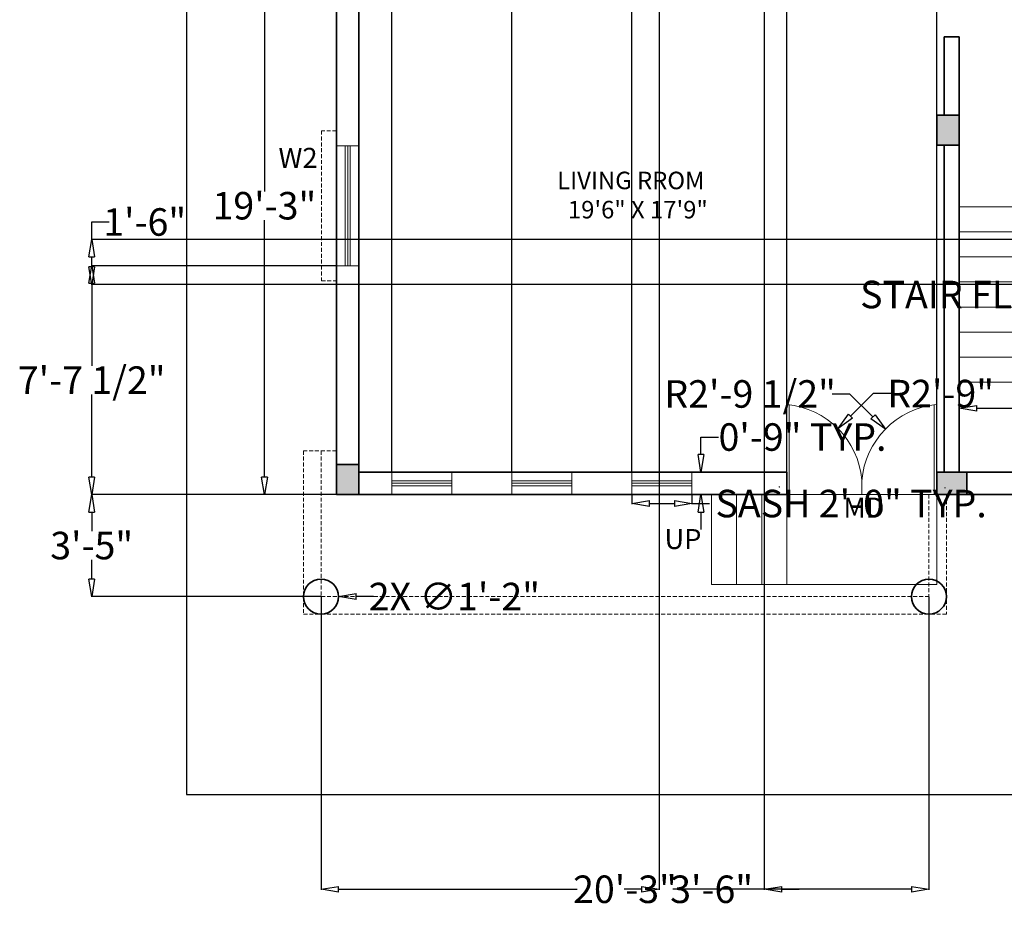
# Model space of a CAD drawing. Units: inches. Extents: x 668 to 1552, y 994 to 1684.
# Tile 1 of 4: x 668 to 1061, y 994 to 1349. Entities that reach past the tile are written whole.
import ezdxf

# ---------------------------------------------------------------- set-up
doc = ezdxf.new("R2010")
doc.units = ezdxf.units.IN
doc.header["$LTSCALE"] = 2.5
doc.header["$MEASUREMENT"] = 0
doc.linetypes.add('HIDDEN', pattern=[0.375, 0.25, -0.125])
for name, color, linetype, lineweight, true_color in [('A-ANNO-DIMS', 175, 'Continuous', 13, 0x4554a5), ('A-ANNO-TEXT', 52, 'Continuous', 18, 0xc8c92d), ('A-DOOR', 152, 'Continuous', 18, 0x2776bb), ('A-FLOR-STRS', 165, 'Continuous', 18, 0x5e67af)]:
    doc.layers.add(name, color=color, linetype=linetype, lineweight=lineweight, true_color=true_color)
for name, color, linetype, lineweight in [('A-AREA-IDEN', 2, 'Continuous', 18), ('A-COLS', 7, 'Continuous', 35), ('A-COLS-PATT', 1, 'Continuous', 13), ('A-GLAZ', 4, 'Continuous', 18), ('A-ROOF-OVHD', 82, 'HIDDEN', 13), ('A-WALL', 7, 'Continuous', 35), ('C-PROP', 1, 'Continuous', 25), ('sajjas', 210, 'HIDDEN', 13)]:
    doc.layers.add(name, color=color, linetype=linetype, lineweight=lineweight)
doc.styles.get("Standard").update_dxf_attribs({"font": 'arial.ttf'})
doc.dimstyles.get("Standard").update_dxf_attribs({"dimtxt": 11, "dimasz": 7, "dimexe": 0.18, "dimexo": 0.0625, "dimgap": 0.09, "dimtad": 0, "dimtih": 1, "dimtoh": 1, "dimdec": 0, "dimzin": 0, "dimdsep": 46, "dimlunit": 3, "dimtxsty": 'Standard', "dimblk": 'CLOSEDBLANK', "dimcen": 0.09, "dimadec": 0, "dimazin": 0, "dimtfac": 1, "dimtdec": 0, "dimtofl": 0, "dimtmove": 0, "dimatfit": 3, "dimldrblk": 'CLOSEDBLANK', "dimfxl": 1, "dimtolj": 1, "dimtzin": 0, "dimarcsym": 0})

# ---------------------------------------------------------------- blocks, each defined once
blk = doc.blocks.new('_ClosedBlank')
at = {"color": 0, "linetype": 'ByBlock', "lineweight": -2}
for p, q in [((-1, 0.167), (0, 0)), ((-1, 0.167), (-1, -0.167)), ((0, 0), (-1, -0.167))]:
    blk.add_line(p, q, dxfattribs=at)
blk = doc.blocks.new('*D5')
at = {"layer": 'A-ANNO-DIMS', "color": 0, "lineweight": -2, "ltscale": 2.5, "transparency": 16777216}
for p, q in [((794.3, 1390.35), (765.38, 1390.35)), ((765.56, 1383.35), (765.56, 1280.56)), ((765.56, 1166.35), (765.56, 1269.14)), ((794.3, 1159.35), (765.38, 1159.35))]:
    blk.add_line(p, q, dxfattribs=at)
at = {"layer": 'Defpoints', "color": 0, "ltscale": 2.5, "transparency": 16777216}
for p in [(765.56, 1390.35), (794.36, 1390.35), (794.36, 1159.35)]:
    blk.add_point(p, dxfattribs=at)
at = {"layer": 'A-ANNO-DIMS', "color": 0, "lineweight": -2, "ltscale": 2.5, "transparency": 16777216, "xscale": 7, "yscale": 7, "zscale": 7}
for p, rotation in [((765.56, 1390.35), 90), ((765.56, 1159.35), 270)]:
    blk.add_blockref('_ClosedBlank', p, dxfattribs=dict(at, rotation=rotation))
at = {"layer": 'A-ANNO-DIMS', "color": 0, "ltscale": 2.5, "transparency": 16777216, "insert": (765.56, 1274.85), "char_height": 11, "attachment_point": 5}
blk.add_mtext('\\A1;19\'-3"', dxfattribs=at)
blk = doc.blocks.new('WIN-48')
for p, q in [((0, 9), (48, 9)), ((0, 9), (0, 0)), ((48, 9), (48, 0)), ((48, 5.5), (0, 5.5)), ((48, 4.5), (0, 4.5)), ((48, 3.5), (0, 3.5)), ((0, 0), (48, 0))]:
    blk.add_line(p, q)
blk = doc.blocks.new('WIN-PORCH-24')
for p, q in [((0, 9), (0, 0)), ((0, 9), (24, 9)), ((0, 0), (0, 9)), ((24, 9), (24, 0)), ((24, 5.5), (0.04, 5.5)), ((24, 4.5), (0.04, 4.5)), ((24, 0), (0, 0)), ((24, 3.5), (0.04, 3.5))]:
    blk.add_line(p, q)
blk = doc.blocks.new('SAJJA-60')
at = {"ltscale": 2.5}
blk.add_lwpolyline([(6, 6), (0, 6), (0, 0), (54, 0), (60, 0), (60, 6), (54, 6)], dxfattribs=at)
blk = doc.blocks.new('STAIR-FLIGHT-37')
at = {"ltscale": 2.5}
for p, q in [((0, 70), (37, 70)), ((37, 0), (37, 70)), ((0, 60), (37, 60)), ((0, 50), (37, 50)), ((0, 40), (37, 40)), ((0, 30), (37, 30)), ((0, 20), (37, 20)), ((0, 10), (37, 10))]:
    blk.add_line(p, q, dxfattribs=at)
blk = doc.blocks.new('COL-ROUND-14')
at = {"ltscale": 2.5}
blk.add_circle((7, 7), 7, dxfattribs=at)
blk = doc.blocks.new('*D28')
at = {"layer": 'A-ANNO-DIMS', "color": 0, "lineweight": -2, "ltscale": 2.5, "transparency": 16777216}
for p, q in [((912.48, 1159.29), (912.48, 1155.57)), ((936.48, 1159.29), (936.48, 1155.57)), ((919.48, 1155.75), (929.48, 1155.75)), ((936.48, 1155.75), (943.48, 1155.75))]:
    blk.add_line(p, q, dxfattribs=at)
at = {"layer": 'Defpoints', "color": 0, "ltscale": 2.5, "transparency": 16777216}
for p in [(912.48, 1159.35), (936.48, 1159.35), (936.48, 1155.75)]:
    blk.add_point(p, dxfattribs=at)
at = {"layer": 'A-ANNO-DIMS', "color": 0, "lineweight": -2, "ltscale": 2.5, "transparency": 16777216, "xscale": 7, "yscale": 7, "zscale": 7, "rotation": 180}
blk.add_blockref('_ClosedBlank', (912.48, 1155.75), dxfattribs=at)
at = {"layer": 'A-ANNO-DIMS', "color": 0, "lineweight": -2, "ltscale": 2.5, "transparency": 16777216, "xscale": 7, "yscale": 7, "zscale": 7}
blk.add_blockref('_ClosedBlank', (936.48, 1155.75), dxfattribs=at)
at = {"layer": 'A-ANNO-DIMS', "color": 0, "ltscale": 2.5, "transparency": 16777216, "insert": (1000.13, 1155.75), "char_height": 11, "attachment_point": 5}
blk.add_mtext('\\A1;SASH 2\'-0" TYP.', dxfattribs=at)
blk = doc.blocks.new('*D29')
at = {"layer": 'A-ANNO-DIMS', "color": 0, "lineweight": -2, "ltscale": 2.5, "transparency": 16777216}
for p, q in [((940.08, 1175.35), (940.08, 1182.35)), ((940.08, 1182.35), (947.08, 1182.35)), ((936.54, 1168.35), (940.26, 1168.35)), ((936.54, 1159.35), (940.26, 1159.35)), ((940.08, 1152.35), (940.08, 1145.35))]:
    blk.add_line(p, q, dxfattribs=at)
at = {"layer": 'Defpoints', "color": 0, "ltscale": 2.5, "transparency": 16777216}
for p in [(936.48, 1168.35), (940.08, 1168.35), (936.48, 1159.35)]:
    blk.add_point(p, dxfattribs=at)
at = {"layer": 'A-ANNO-DIMS', "color": 0, "lineweight": -2, "ltscale": 2.5, "transparency": 16777216, "xscale": 7, "yscale": 7, "zscale": 7}
for p, rotation in [((940.08, 1168.35), 270), ((940.08, 1159.35), 90)]:
    blk.add_blockref('_ClosedBlank', p, dxfattribs=dict(at, rotation=rotation))
at = {"layer": 'A-ANNO-DIMS', "color": 0, "ltscale": 2.5, "transparency": 16777216, "insert": (980.69, 1182.35), "char_height": 11, "attachment_point": 5}
blk.add_mtext('\\A1;0\'-9" TYP.', dxfattribs=at)
blk = doc.blocks.new('*D32')
at = {"layer": 'A-ANNO-DIMS', "color": 0, "lineweight": -2, "ltscale": 2.5, "transparency": 16777216}
for p, q in [((1080.43, 1274.35), (1091.04, 1274.35)), ((1090.86, 1267.35), (1090.86, 1245.13)), ((1090.86, 1211.35), (1090.86, 1233.57)), ((1080.43, 1204.35), (1091.04, 1204.35))]:
    blk.add_line(p, q, dxfattribs=at)
at = {"layer": 'Defpoints', "color": 0, "ltscale": 2.5, "transparency": 16777216}
for p in [(1080.36, 1274.35), (1090.86, 1274.35), (1080.36, 1204.35)]:
    blk.add_point(p, dxfattribs=at)
at = {"layer": 'A-ANNO-DIMS', "color": 0, "lineweight": -2, "ltscale": 2.5, "transparency": 16777216, "xscale": 7, "yscale": 7, "zscale": 7}
for p, rotation in [((1090.86, 1274.35), 90), ((1090.86, 1204.35), 270)]:
    blk.add_blockref('_ClosedBlank', p, dxfattribs=dict(at, rotation=rotation))
at = {"layer": 'A-ANNO-DIMS', "color": 0, "ltscale": 2.5, "transparency": 16777216, "insert": (1090.86, 1239.35), "char_height": 11, "attachment_point": 5}
blk.add_mtext('\\A1;STAIR FLIGHT 5\'-10" TYP.', dxfattribs=at)
blk = doc.blocks.new('*D33')
at = {"layer": 'A-ANNO-DIMS', "color": 0, "lineweight": -2, "ltscale": 2.5, "transparency": 16777216}
for p, q in [((1043.36, 1204.29), (1043.36, 1193.67)), ((1080.36, 1204.29), (1080.36, 1193.67)), ((1050.36, 1193.85), (1073.36, 1193.85)), ((1080.36, 1193.85), (1087.36, 1193.85))]:
    blk.add_line(p, q, dxfattribs=at)
at = {"layer": 'Defpoints', "color": 0, "ltscale": 2.5, "transparency": 16777216}
for p in [(1043.36, 1204.35), (1080.36, 1204.35), (1080.36, 1193.85)]:
    blk.add_point(p, dxfattribs=at)
at = {"layer": 'A-ANNO-DIMS', "color": 0, "lineweight": -2, "ltscale": 2.5, "transparency": 16777216, "xscale": 7, "yscale": 7, "zscale": 7, "rotation": 180}
blk.add_blockref('_ClosedBlank', (1043.36, 1193.85), dxfattribs=at)
at = {"layer": 'A-ANNO-DIMS', "color": 0, "lineweight": -2, "ltscale": 2.5, "transparency": 16777216, "xscale": 7, "yscale": 7, "zscale": 7}
blk.add_blockref('_ClosedBlank', (1080.36, 1193.85), dxfattribs=at)
at = {"layer": 'A-ANNO-DIMS', "color": 0, "ltscale": 2.5, "transparency": 16777216, "insert": (1120.97, 1193.85), "char_height": 11, "attachment_point": 5}
blk.add_mtext('\\A1;3\'-1" TYP.', dxfattribs=at)
blk = doc.blocks.new('*D35')
at = {"layer": 'A-ANNO-DIMS', "color": 0, "lineweight": -2, "ltscale": 2.5, "transparency": 16777216}
for p, q in [((788.19, 1118.49), (788.19, 1001.32)), ((1031.23, 1118.49), (1031.23, 1001.32)), ((795.19, 1001.5), (890.63, 1001.5)), ((1024.23, 1001.5), (928.79, 1001.5))]:
    blk.add_line(p, q, dxfattribs=at)
at = {"layer": 'Defpoints', "color": 0, "ltscale": 2.5, "transparency": 16777216}
for p in [(788.19, 1118.56), (1031.23, 1118.56), (1031.23, 1001.5)]:
    blk.add_point(p, dxfattribs=at)
at = {"layer": 'A-ANNO-DIMS', "color": 0, "lineweight": -2, "ltscale": 2.5, "transparency": 16777216, "xscale": 7, "yscale": 7, "zscale": 7, "rotation": 180}
blk.add_blockref('_ClosedBlank', (788.19, 1001.5), dxfattribs=at)
at = {"layer": 'A-ANNO-DIMS', "color": 0, "lineweight": -2, "ltscale": 2.5, "transparency": 16777216, "xscale": 7, "yscale": 7, "zscale": 7}
blk.add_blockref('_ClosedBlank', (1031.23, 1001.5), dxfattribs=at)
at = {"layer": 'A-ANNO-DIMS', "color": 0, "ltscale": 2.5, "transparency": 16777216, "insert": (909.71, 1001.5), "char_height": 11, "attachment_point": 5}
blk.add_mtext('\\A1;20\'-3"', dxfattribs=at)
blk = doc.blocks.new('*D36')
at = {"layer": 'A-ANNO-DIMS', "color": 0, "lineweight": -2, "ltscale": 2.5, "transparency": 16777216}
for p, q in [((794.3, 1159.35), (696.33, 1159.35)), ((696.51, 1152.35), (696.51, 1144.66)), ((696.51, 1125.56), (696.51, 1133.24)), ((788.13, 1118.56), (696.33, 1118.56))]:
    blk.add_line(p, q, dxfattribs=at)
at = {"layer": 'Defpoints', "color": 0, "ltscale": 2.5, "transparency": 16777216}
for p in [(794.36, 1159.35), (696.51, 1118.56), (788.19, 1118.56)]:
    blk.add_point(p, dxfattribs=at)
at = {"layer": 'A-ANNO-DIMS', "color": 0, "lineweight": -2, "ltscale": 2.5, "transparency": 16777216, "xscale": 7, "yscale": 7, "zscale": 7}
for p, rotation in [((696.51, 1159.35), 90), ((696.51, 1118.56), 270)]:
    blk.add_blockref('_ClosedBlank', p, dxfattribs=dict(at, rotation=rotation))
at = {"layer": 'A-ANNO-DIMS', "color": 0, "ltscale": 2.5, "transparency": 16777216, "insert": (696.51, 1138.95), "char_height": 11, "attachment_point": 5}
blk.add_mtext('\\A1;3\'-5"', dxfattribs=at)
blk = doc.blocks.new('*D37')
at = {"layer": 'A-ANNO-DIMS', "color": 0, "lineweight": -2, "ltscale": 2.5, "transparency": 16777216}
for p, q in [((974.36, 1168.41), (974.36, 1677.38)), ((981.36, 1677.2), (989.65, 1677.2)), ((1027.36, 1677.2), (1019.07, 1677.2)), ((1034.36, 1168.41), (1034.36, 1677.38))]:
    blk.add_line(p, q, dxfattribs=at)
at = {"layer": 'Defpoints', "color": 0, "ltscale": 2.5, "transparency": 16777216}
for p in [(1034.36, 1677.2), (974.36, 1168.35), (1034.36, 1168.35)]:
    blk.add_point(p, dxfattribs=at)
at = {"layer": 'A-ANNO-DIMS', "color": 0, "lineweight": -2, "ltscale": 2.5, "transparency": 16777216, "xscale": 7, "yscale": 7, "zscale": 7, "rotation": 180}
blk.add_blockref('_ClosedBlank', (974.36, 1677.2), dxfattribs=at)
at = {"layer": 'A-ANNO-DIMS', "color": 0, "lineweight": -2, "ltscale": 2.5, "transparency": 16777216, "xscale": 7, "yscale": 7, "zscale": 7}
blk.add_blockref('_ClosedBlank', (1034.36, 1677.2), dxfattribs=at)
at = {"layer": 'A-ANNO-DIMS', "color": 0, "ltscale": 2.5, "transparency": 16777216, "insert": (1004.36, 1677.2), "char_height": 11, "attachment_point": 5}
blk.add_mtext('\\A1;5\'-0"', dxfattribs=at)
blk = doc.blocks.new('*D38')
at = {"layer": 'A-ANNO-DIMS', "color": 0, "lineweight": -2, "ltscale": 2.5, "transparency": 16777216}
for p, q in [((923.362549, 1570.287512), (923.362549, 1001.320012)), ((965.362549, 1570.287512), (965.362549, 1001.320012)), ((916.362549, 1001.500012), (909.362549, 1001.500012)), ((972.362549, 1001.500012), (979.362549, 1001.500012))]:
    blk.add_line(p, q, dxfattribs=at)
at = {"layer": 'Defpoints', "color": 0, "ltscale": 2.5, "transparency": 16777216}
for p in [(923.362549, 1570.350012), (965.362549, 1570.350012), (965.362549, 1001.500012)]:
    blk.add_point(p, dxfattribs=at)
at = {"layer": 'A-ANNO-DIMS', "color": 0, "lineweight": -2, "ltscale": 2.5, "transparency": 16777216, "xscale": 7, "yscale": 7, "zscale": 7}
blk.add_blockref('_ClosedBlank', (923.362549, 1001.500012), dxfattribs=at)
at = {"layer": 'A-ANNO-DIMS', "color": 0, "lineweight": -2, "ltscale": 2.5, "transparency": 16777216, "xscale": 7, "yscale": 7, "zscale": 7, "rotation": 180}
blk.add_blockref('_ClosedBlank', (965.362549, 1001.500012), dxfattribs=at)
at = {"layer": 'A-ANNO-DIMS', "color": 0, "ltscale": 2.5, "transparency": 16777216, "insert": (944.362549, 1001.500012), "char_height": 11, "attachment_point": 5}
blk.add_mtext('\\A1;3\'-6"', dxfattribs=at)
blk = doc.blocks.new('*D45')
at = {"layer": 'A-ANNO-DIMS', "color": 0, "lineweight": -2, "ltscale": 2.5, "transparency": 16777216}
for p, q in [((794.3, 1250.85), (696.33, 1250.85)), ((696.51, 1243.85), (696.51, 1210.88)), ((696.51, 1166.35), (696.51, 1199.32)), ((794.3, 1159.35), (696.33, 1159.35))]:
    blk.add_line(p, q, dxfattribs=at)
at = {"layer": 'Defpoints', "color": 0, "ltscale": 2.5, "transparency": 16777216}
for p in [(696.51, 1250.85), (794.36, 1250.85), (794.36, 1159.35)]:
    blk.add_point(p, dxfattribs=at)
at = {"layer": 'A-ANNO-DIMS', "color": 0, "lineweight": -2, "ltscale": 2.5, "transparency": 16777216, "xscale": 7, "yscale": 7, "zscale": 7}
for p, rotation in [((696.51, 1250.85), 90), ((696.51, 1159.35), 270)]:
    blk.add_blockref('_ClosedBlank', p, dxfattribs=dict(at, rotation=rotation))
at = {"layer": 'A-ANNO-DIMS', "color": 0, "ltscale": 2.5, "transparency": 16777216, "insert": (696.51, 1205.1), "char_height": 11, "attachment_point": 5}
blk.add_mtext('\\A1;7\'-7 1/2"', dxfattribs=at)
blk = doc.blocks.new('*D46')
at = {"layer": 'A-ANNO-DIMS', "color": 0, "lineweight": -2, "ltscale": 2.5, "transparency": 16777216}
for p, q in [((796.36, 1677.2), (789.36, 1677.2)), ((803.36, 1168.41), (803.36, 1677.38)), ((816.48, 1168.41), (816.48, 1677.38)), ((823.48, 1677.2), (830.48, 1677.2))]:
    blk.add_line(p, q, dxfattribs=at)
at = {"layer": 'Defpoints', "color": 0, "ltscale": 2.5, "transparency": 16777216}
for p in [(816.48, 1677.2), (803.36, 1168.35), (816.48, 1168.35)]:
    blk.add_point(p, dxfattribs=at)
at = {"layer": 'A-ANNO-DIMS', "color": 0, "lineweight": -2, "ltscale": 2.5, "transparency": 16777216, "xscale": 7, "yscale": 7, "zscale": 7}
blk.add_blockref('_ClosedBlank', (803.36, 1677.2), dxfattribs=at)
at = {"layer": 'A-ANNO-DIMS', "color": 0, "lineweight": -2, "ltscale": 2.5, "transparency": 16777216, "xscale": 7, "yscale": 7, "zscale": 7, "rotation": 180}
blk.add_blockref('_ClosedBlank', (816.48, 1677.2), dxfattribs=at)
at = {"layer": 'A-ANNO-DIMS', "color": 0, "ltscale": 2.5, "transparency": 16777216, "insert": (844.67, 1677.2), "char_height": 11, "attachment_point": 5}
blk.add_mtext('\\A1;1\'-1"', dxfattribs=at)
blk = doc.blocks.new('*D47')
at = {"layer": 'A-ANNO-DIMS', "color": 0, "lineweight": -2, "ltscale": 2.5, "transparency": 16777216}
for p, q in [((816.48, 1168.41), (816.48, 1677.38)), ((823.48, 1677.2), (825.55, 1677.2)), ((857.48, 1677.2), (855.41, 1677.2)), ((864.48, 1168.41), (864.48, 1677.38))]:
    blk.add_line(p, q, dxfattribs=at)
at = {"layer": 'Defpoints', "color": 0, "ltscale": 2.5, "transparency": 16777216}
for p in [(864.48, 1677.2), (816.48, 1168.35), (864.48, 1168.35)]:
    blk.add_point(p, dxfattribs=at)
at = {"layer": 'A-ANNO-DIMS', "color": 0, "lineweight": -2, "ltscale": 2.5, "transparency": 16777216, "xscale": 7, "yscale": 7, "zscale": 7, "rotation": 180}
blk.add_blockref('_ClosedBlank', (816.48, 1677.2), dxfattribs=at)
at = {"layer": 'A-ANNO-DIMS', "color": 0, "lineweight": -2, "ltscale": 2.5, "transparency": 16777216, "xscale": 7, "yscale": 7, "zscale": 7}
blk.add_blockref('_ClosedBlank', (864.48, 1677.2), dxfattribs=at)
at = {"layer": 'A-ANNO-DIMS', "color": 0, "ltscale": 2.5, "transparency": 16777216, "insert": (840.48, 1677.2), "char_height": 11, "attachment_point": 5}
blk.add_mtext('\\A1;4\'-0"', dxfattribs=at)
blk = doc.blocks.new('*D48')
at = {"layer": 'A-ANNO-DIMS', "color": 0, "lineweight": -2, "ltscale": 2.5, "transparency": 16777216}
for p, q in [((864.48, 1168.41), (864.48, 1677.38)), ((871.48, 1677.2), (873.55, 1677.2)), ((905.48, 1677.2), (903.41, 1677.2)), ((912.48, 1168.41), (912.48, 1677.38))]:
    blk.add_line(p, q, dxfattribs=at)
at = {"layer": 'Defpoints', "color": 0, "ltscale": 2.5, "transparency": 16777216}
for p in [(912.48, 1677.2), (864.48, 1168.35), (912.48, 1168.35)]:
    blk.add_point(p, dxfattribs=at)
at = {"layer": 'A-ANNO-DIMS', "color": 0, "lineweight": -2, "ltscale": 2.5, "transparency": 16777216, "xscale": 7, "yscale": 7, "zscale": 7, "rotation": 180}
blk.add_blockref('_ClosedBlank', (864.48, 1677.2), dxfattribs=at)
at = {"layer": 'A-ANNO-DIMS', "color": 0, "lineweight": -2, "ltscale": 2.5, "transparency": 16777216, "xscale": 7, "yscale": 7, "zscale": 7}
blk.add_blockref('_ClosedBlank', (912.48, 1677.2), dxfattribs=at)
at = {"layer": 'A-ANNO-DIMS', "color": 0, "ltscale": 2.5, "transparency": 16777216, "insert": (888.48, 1677.2), "char_height": 11, "attachment_point": 5}
blk.add_mtext('\\A1;4\'-0"', dxfattribs=at)
blk = doc.blocks.new('*D51')
at = {"layer": 'A-ANNO-DIMS', "color": 0, "lineweight": -2, "ltscale": 2.5, "transparency": 16777216}
for p, q in [((696.51, 1261.35), (696.51, 1268.35)), ((696.51, 1268.35), (703.51, 1268.35)), ((1385.3, 1261.35), (696.33, 1261.35)), ((696.51, 1250.35), (696.51, 1254.35)), ((1385.3, 1243.35), (696.33, 1243.35))]:
    blk.add_line(p, q, dxfattribs=at)
at = {"layer": 'Defpoints', "color": 0, "ltscale": 2.5, "transparency": 16777216}
for p in [(696.51, 1261.35), (1385.36, 1261.35), (1385.36, 1243.35)]:
    blk.add_point(p, dxfattribs=at)
at = {"layer": 'A-ANNO-DIMS', "color": 0, "lineweight": -2, "ltscale": 2.5, "transparency": 16777216, "xscale": 7, "yscale": 7, "zscale": 7}
for p, rotation in [((696.51, 1261.35), 90), ((696.51, 1243.35), 270)]:
    blk.add_blockref('_ClosedBlank', p, dxfattribs=dict(at, rotation=rotation))
at = {"layer": 'A-ANNO-DIMS', "color": 0, "ltscale": 2.5, "transparency": 16777216, "insert": (717.71, 1268.35), "char_height": 11, "attachment_point": 5}
blk.add_mtext('\\A1;1\'-6"', dxfattribs=at)
blk = doc.blocks.new('*D52')
at = {"layer": 'A-ANNO-DIMS', "color": 0, "lineweight": -2, "ltscale": 2.5, "transparency": 16777216}
for p, q in [((788.1, 1118.56), (788.28, 1118.56)), ((788.19, 1118.47), (788.19, 1118.65)), ((809.19, 1118.56), (802.19, 1118.56))]:
    blk.add_line(p, q, dxfattribs=at)
at = {"layer": 'Defpoints', "color": 0, "ltscale": 2.5, "transparency": 16777216}
for p in [(781.19, 1118.56), (795.19, 1118.56)]:
    blk.add_point(p, dxfattribs=at)
at = {"layer": 'A-ANNO-DIMS', "color": 0, "lineweight": -2, "ltscale": 2.5, "transparency": 16777216, "xscale": 7, "yscale": 7, "zscale": 7, "rotation": 180.0038470023325}
blk.add_blockref('_ClosedBlank', (795.19, 1118.56), dxfattribs=at)
at = {"layer": 'A-ANNO-DIMS', "color": 0, "ltscale": 2.5, "transparency": 16777216, "insert": (841.51, 1118.56), "char_height": 11, "attachment_point": 5}
blk.add_mtext('\\A1;2X ∅1\'-2"', dxfattribs=at)
blk = doc.blocks.new('*D54')
at = {"layer": 'A-ANNO-DIMS', "color": 0, "lineweight": -2, "ltscale": 2.5, "transparency": 16777216}
for p, q in [((992.53, 1199.58), (999.53, 1199.58)), ((999.53, 1199.58), (1008.85, 1190.43)), ((1037.59, 1162.09), (1037.77, 1162.09)), ((1037.68, 1162), (1037.68, 1162.18))]:
    blk.add_line(p, q, dxfattribs=at)
at = {"layer": 'Defpoints', "color": 0, "ltscale": 2.5, "transparency": 16777216}
for p in [(1013.84, 1185.52), (1037.68, 1162.09)]:
    blk.add_point(p, dxfattribs=at)
at = {"layer": 'A-ANNO-DIMS', "color": 0, "lineweight": -2, "ltscale": 2.5, "transparency": 16777216, "xscale": 7, "yscale": 7, "zscale": 7, "rotation": 315.4942682278038}
blk.add_blockref('_ClosedBlank', (1013.84, 1185.52), dxfattribs=at)
at = {"layer": 'A-ANNO-DIMS', "color": 0, "ltscale": 2.5, "transparency": 16777216, "insert": (959.74, 1199.58), "char_height": 11, "attachment_point": 5}
blk.add_mtext('\\A1;R2\'-9 1/2"', dxfattribs=at)
blk = doc.blocks.new('*D55')
at = {"layer": 'A-ANNO-DIMS', "color": 0, "lineweight": -2, "ltscale": 2.5, "transparency": 16777216}
for p, q in [((1008.94, 1199.73), (999.85, 1190.68)), ((1015.94, 1199.73), (1008.94, 1199.73)), ((971.37, 1162.43), (971.55, 1162.43)), ((971.46, 1162.34), (971.46, 1162.52))]:
    blk.add_line(p, q, dxfattribs=at)
at = {"layer": 'Defpoints', "color": 0, "ltscale": 2.5, "transparency": 16777216}
for p in [(994.88, 1185.74), (971.46, 1162.43)]:
    blk.add_point(p, dxfattribs=at)
at = {"layer": 'A-ANNO-DIMS', "color": 0, "lineweight": -2, "ltscale": 2.5, "transparency": 16777216, "xscale": 7, "yscale": 7, "zscale": 7, "rotation": 224.8569639041419}
blk.add_blockref('_ClosedBlank', (994.88, 1185.74), dxfattribs=at)
at = {"layer": 'A-ANNO-DIMS', "color": 0, "ltscale": 2.5, "transparency": 16777216, "insert": (1035.92, 1199.73), "char_height": 11, "attachment_point": 5}
blk.add_mtext('\\A1;R2\'-9"', dxfattribs=at)

msp = doc.modelspace()

# ---------------------------------------------------------------- hatches: boundary and pattern name
at = {"layer": 'A-COLS-PATT'}
h = msp.add_hatch(color=256, dxfattribs=at)
h.dxf.hatch_style = 1
h.paths.add_polyline_path([(803.36, 1390.35), (794.36, 1390.35), (794.36, 1378.35), (803.36, 1378.35)])
h.paths.add_polyline_path([(1117.36, 1393.35), (1108.36, 1393.35), (1108.36, 1381.35), (1117.36, 1381.35)])
h.paths.add_polyline_path([(1255.36, 1390.35), (1243.36, 1390.35), (1243.36, 1381.35), (1255.36, 1381.35)])
h.paths.add_polyline_path([(1394.36, 1390.35), (1382.36, 1390.35), (1382.36, 1381.35), (1394.36, 1381.35)])
h.paths.add_polyline_path([(1394.36, 1579.35), (1385.36, 1579.35), (1385.36, 1567.35), (1394.36, 1567.35)])
h.paths.add_polyline_path([(1253.36, 1579.35), (1241.36, 1579.35), (1241.36, 1570.35), (1253.36, 1570.35)])
h.paths.add_polyline_path([(1115.36, 1579.35), (1103.36, 1579.35), (1103.36, 1570.35), (1115.36, 1570.35)])
h.paths.add_polyline_path([(923.36, 1579.35), (914.36, 1579.35), (914.36, 1567.35), (923.36, 1567.35)])
h.paths.add_polyline_path([(926.36, 1390.35), (914.36, 1390.35), (914.36, 1381.35), (926.36, 1381.35)])
h.paths.add_polyline_path([(1394.36, 1243.35), (1382.36, 1243.35), (1382.36, 1234.35), (1394.36, 1234.35)])
h.paths.add_polyline_path([(1277.36, 1342.35), (1265.36, 1342.35), (1265.36, 1333.35), (1277.36, 1333.35)])
h.paths.add_polyline_path([(1130.36, 1311.02), (1121.36, 1311.02), (1121.36, 1299.02), (1130.36, 1299.02)])
h.paths.add_polyline_path([(1043.36, 1311.02), (1034.36, 1311.02), (1034.36, 1299.02), (1043.36, 1299.02)])
h.paths.add_polyline_path([(803.36, 1171.35), (794.36, 1171.35), (794.36, 1159.35), (803.36, 1159.35)])
h.paths.add_polyline_path([(1046.36, 1168.35), (1034.36, 1168.35), (1034.36, 1159.35), (1046.36, 1159.35)])
h.paths.add_polyline_path([(1133.36, 1168.35), (1121.36, 1168.35), (1121.36, 1159.35), (1133.36, 1159.35)])
h.paths.add_polyline_path([(1277.36, 1168.35), (1265.36, 1168.35), (1265.36, 1159.35), (1277.36, 1159.35)])

# ---------------------------------------------------------------- linework, layer by layer
at = {"layer": 'A-COLS'}
for points in [[(1034.36, 1299.02), (1043.36, 1299.02), (1043.36, 1311.02), (1034.36, 1311.02)], [(794.36, 1159.35), (803.36, 1159.35), (803.36, 1171.35), (794.36, 1171.35)], [(1046.36, 1159.35), (1046.36, 1168.35), (1034.36, 1168.35), (1034.36, 1159.35)]]:
    msp.add_lwpolyline(points, close=True, dxfattribs=at)
at = {"layer": 'A-DOOR'}
for p, q in [((974.36, 1159.35), (974.36, 1195.35)), ((975.36, 1159.35), (975.36, 1195.35)), ((1033.36, 1159.35), (1033.36, 1195.35)), ((1034.36, 1159.35), (1034.36, 1195.35)), ((1004.36, 1159.35), (1004.36, 1165.51)), ((974.36, 1159.35), (1034.36, 1159.35))]:
    msp.add_line(p, q, dxfattribs=at)
for centre, radius, start, end in [((971.46, 1162.43), 33.05, 4.7571, 84.9567), ((1037.68, 1162.09), 33.43, 95.6889, 175.3)]:
    msp.add_arc(centre, radius, start, end, dxfattribs=at)
at = {"layer": 'A-FLOR-STRS', "ltscale": 2.5}
for p, q in [((1043.36, 1204.35), (1121.36, 1204.35)), ((944.36, 1123.35), (944.36, 1159.35)), ((954.36, 1123.35), (954.36, 1159.35)), ((964.36, 1123.35), (964.36, 1159.35)), ((974.36, 1123.35), (974.36, 1159.35)), ((1034.36, 1159.35), (1034.36, 1123.35)), ((974.36, 1123.35), (944.36, 1123.35)), ((1034.36, 1123.35), (974.36, 1123.35))]:
    msp.add_line(p, q, dxfattribs=at)
at = {"layer": 'A-ROOF-OVHD', "ltscale": 2.5}
for p, q in [((794.36, 1176.85), (781.19, 1176.85)), ((781.19, 1176.85), (781.19, 1111.56)), ((788.19, 1176.85), (788.19, 1118.56)), ((1031.23, 1159.35), (1031.23, 1118.56)), ((1038.23, 1159.35), (1038.23, 1111.56)), ((1031.23, 1118.56), (788.19, 1118.56)), ((1038.23, 1111.56), (781.19, 1111.56))]:
    msp.add_line(p, q, dxfattribs=at)
at = {"layer": 'A-WALL'}
for p, q in [((794.36, 1390.35), (794.36, 1159.35)), ((803.36, 1381.35), (803.36, 1168.35)), ((1037.36, 1342.35), (1037.36, 1311.02)), ((1037.36, 1342.35), (1043.36, 1342.35)), ((1043.36, 1342.35), (1043.36, 1168.35)), ((1037.36, 1299.02), (1037.36, 1168.35)), ((803.36, 1168.35), (974.36, 1168.35)), ((974.36, 1168.35), (974.36, 1159.35)), ((1034.36, 1168.35), (1034.36, 1159.35)), ((1034.36, 1168.35), (1037.36, 1168.35)), ((1043.36, 1168.35), (1121.36, 1168.35)), ((794.36, 1159.35), (974.36, 1159.35)), ((1034.36, 1159.35), (1277.36, 1159.35))]:
    msp.add_line(p, q, dxfattribs=at)
at = {"layer": 'C-PROP', "ltscale": 2.5}
for p, q in [((734.36, 1639.35), (734.36, 1039.35)), ((734.36, 1039.35), (1454.36, 1039.35))]:
    msp.add_line(p, q, dxfattribs=at)

# ---------------------------------------------------------------- block references
at = {"layer": 'A-COLS'}
for p in [(781.19, 1111.56), (1024.23, 1111.56)]:
    msp.add_blockref('COL-ROUND-14', p, dxfattribs=at)
at = {"layer": 'A-FLOR-STRS'}
msp.add_blockref('STAIR-FLIGHT-37', (1043.36, 1204.35), dxfattribs=at)
at = {"layer": 'A-GLAZ', "rotation": 270.0000000000007}
msp.add_blockref('WIN-48', (794.36, 1298.85), dxfattribs=at)
at = {"layer": 'A-GLAZ'}
for p in [(816.48, 1159.35), (864.48, 1159.35), (912.48, 1159.35)]:
    msp.add_blockref('WIN-PORCH-24', p, dxfattribs=at)
at = {"layer": 'sajjas', "rotation": 270}
msp.add_blockref('SAJJA-60', (788.36, 1304.85), dxfattribs=at)

# ---------------------------------------------------------------- texts
at = {"layer": 'A-ANNO-TEXT', "ltscale": 2.5, "char_height": 8, "attachment_point": 1}
for s, insert in [('W2', (771.17, 1298)), ('MD', (997.06, 1158.11)), ('UP', (925.5, 1145.56))]:
    msp.add_mtext_dynamic_manual_height_columns(s, width=96.0512, gutter_width=1, heights=[0], dxfattribs=dict(at, insert=insert))
at = {"layer": 'A-AREA-IDEN', "ltscale": 2.5, "insert": (882.62, 1288.46), "char_height": 7, "attachment_point": 1}
msp.add_mtext_dynamic_manual_height_columns('LIVING RROM\\P  19\'6" X 17\'9"', width=108.4664, gutter_width=1, heights=[0], dxfattribs=at)

# ---------------------------------------------------------------- dimensions: what is measured, and where the dimension line sits
at = {"layer": 'A-ANNO-DIMS', "ltscale": 2.5}
for base, p1, p2, picture, middle in [((816.48, 1677.2), (803.36, 1168.35), (816.48, 1168.35), '*D46', (844.67, 1677.2)), ((864.48, 1677.2), (816.48, 1168.35), (864.48, 1168.35), '*D47', (840.48, 1677.2)), ((912.48, 1677.2), (864.48, 1168.35), (912.48, 1168.35), '*D48', (888.48, 1677.2)), ((1034.36, 1677.2), (974.36, 1168.35), (1034.36, 1168.35), '*D37', (1004.36, 1677.2)), ((965.36, 1001.5), (923.36, 1570.35), (965.36, 1570.35), '*D38', (944.36, 1001.5)), ((1031.23, 1001.5), (788.19, 1118.56), (1031.23, 1118.56), '*D35', (909.71, 1001.5))]:
    dim = msp.add_linear_dim(base=base, p1=p1, p2=p2, dimstyle='Standard', override={"dimdec": 1, "dimlfac": 1, "dimrnd": 0, "dimzin": 1, "dimdsep": 46, "dimlunit": 4, "dimfrac": 2}, dxfattribs=at)
    dim.commit()
    dim.dimension.update_dxf_attribs({"geometry": picture, "text_midpoint": middle})
for base, p1, p2, override, picture, middle in [((765.56, 1390.35), (794.36, 1159.35), (794.36, 1390.35), {"dimclrd": 0, "dimclre": 0, "dimclrt": 0}, '*D5', (765.56, 1274.85)), ((696.51, 1261.35), (1385.36, 1243.35), (1385.36, 1261.35), {"dimdec": 1, "dimlfac": 1, "dimrnd": 0, "dimzin": 1, "dimdsep": 46, "dimlunit": 4, "dimfrac": 2}, '*D51', (717.71, 1268.35)), ((696.51, 1250.85), (794.36, 1159.35), (794.36, 1250.85), {"dimdec": 1, "dimlfac": 1, "dimrnd": 0, "dimzin": 1, "dimdsep": 46, "dimlunit": 4, "dimfrac": 2}, '*D45', (696.51, 1205.1)), ((696.51, 1118.56), (794.36, 1159.35), (788.19, 1118.56), {"dimdec": 1, "dimlfac": 1, "dimrnd": 0, "dimzin": 1, "dimdsep": 46, "dimlunit": 4, "dimfrac": 2}, '*D36', (696.51, 1138.95))]:
    dim = msp.add_linear_dim(base=base, p1=p1, p2=p2, angle=90, dimstyle='Standard', override=override, dxfattribs=at)
    dim.commit()
    dim.dimension.update_dxf_attribs({"geometry": picture, "text_midpoint": middle})
for base, p1, p2, text, picture, middle in [((1090.86, 1274.35), (1080.36, 1204.35), (1080.36, 1274.35), 'STAIR FLIGHT <> TYP.', '*D32', (1090.86, 1239.35)), ((940.08, 1168.35), (936.48, 1159.35), (936.48, 1168.35), '<> TYP.', '*D29', (980.69, 1182.35))]:
    dim = msp.add_linear_dim(base=base, p1=p1, p2=p2, angle=90, text=text, dimstyle='Standard', override={"dimdec": 1, "dimlfac": 1, "dimrnd": 0, "dimzin": 1, "dimdsep": 46, "dimlunit": 4, "dimfrac": 2}, dxfattribs=at)
    dim.commit()
    dim.dimension.update_dxf_attribs({"geometry": picture, "text_midpoint": middle})
for center, mpoint, picture, middle in [((1037.68, 1162.09), (1013.84, 1185.52), '*D54', (959.74, 1199.58)), ((971.46, 1162.43), (994.88, 1185.74), '*D55', (1035.92, 1199.73))]:
    dim = msp.add_radius_dim(center=center, mpoint=mpoint, dimstyle='Standard', override={"dimdec": 1, "dimlfac": 1, "dimrnd": 0, "dimzin": 1, "dimdsep": 46, "dimlunit": 4, "dimfrac": 2}, dxfattribs=at)
    dim.commit()
    dim.dimension.update_dxf_attribs({"geometry": picture, "text_midpoint": middle, "dimtype": 164})
for base, p1, p2, text, picture, middle in [((1080.36, 1193.85), (1043.36, 1204.35), (1080.36, 1204.35), '<> TYP.', '*D33', (1120.97, 1193.85)), ((936.48, 1155.75), (912.48, 1159.35), (936.48, 1159.35), 'SASH <> TYP.', '*D28', (1000.13, 1155.75))]:
    dim = msp.add_linear_dim(base=base, p1=p1, p2=p2, text=text, dimstyle='Standard', override={"dimdec": 1, "dimlfac": 1, "dimrnd": 0, "dimzin": 1, "dimdsep": 46, "dimlunit": 4, "dimfrac": 2}, dxfattribs=at)
    dim.commit()
    dim.dimension.update_dxf_attribs({"geometry": picture, "text_midpoint": middle})
dim = msp.add_diameter_dim_2p(p1=(781.19, 1118.56), p2=(795.19, 1118.56), text='2X <>', dimstyle='Standard', override={"dimdec": 1, "dimlfac": 1, "dimrnd": 0, "dimzin": 1, "dimdsep": 46, "dimlunit": 4, "dimfrac": 2}, dxfattribs=at)
dim.commit()
dim.dimension.update_dxf_attribs({"geometry": '*D52', "text_midpoint": (809.19, 1118.56), "dimtype": 163})

doc.saveas('drawing.dxf')
